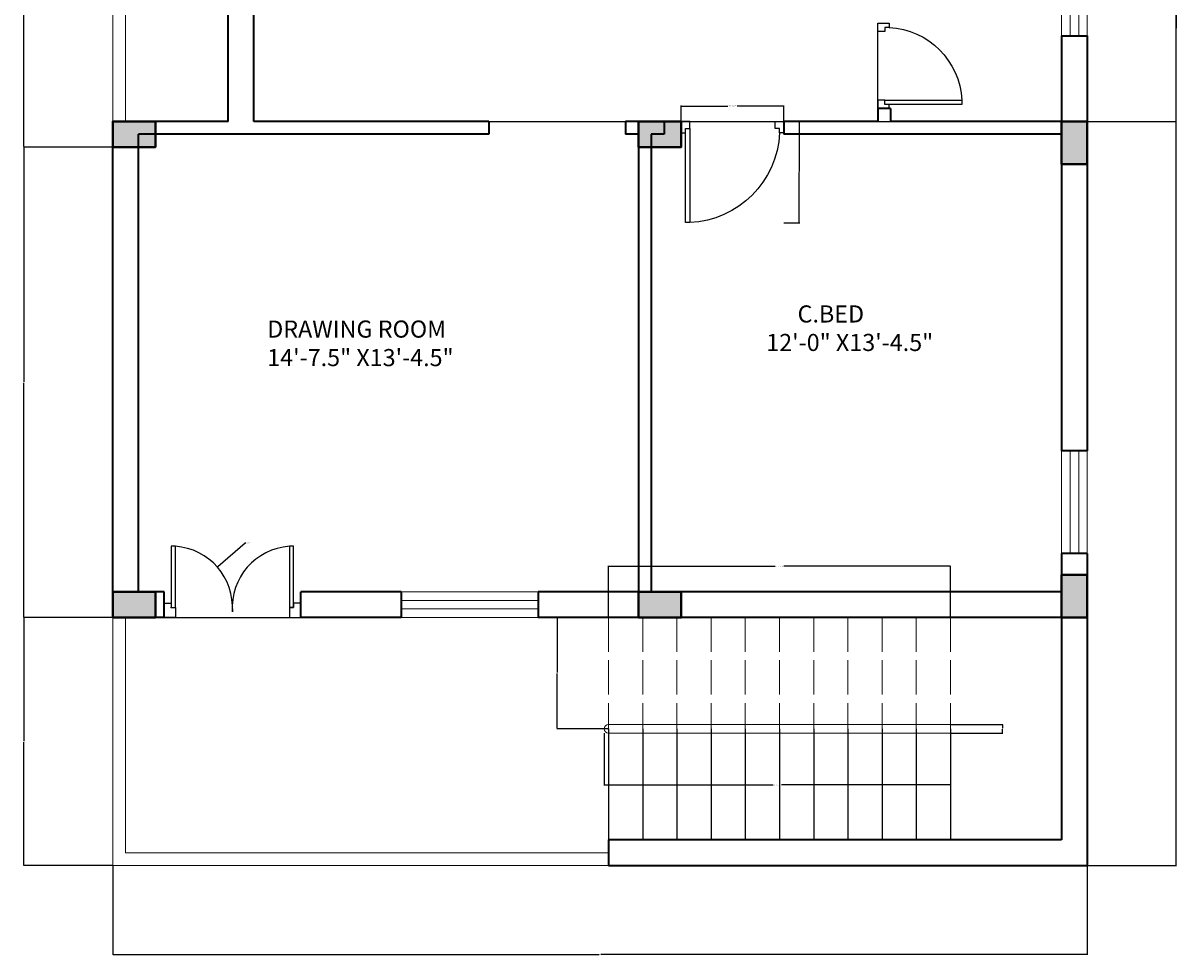
# Model space of a CAD drawing. Units: inches. Extents: x 810 to 2232, y 728 to 1827.
# Tile 5 of 6: x 1827 to 2232, y 1100 to 1426. Entities that reach past the tile are written whole.
import ezdxf

# ---------------------------------------------------------------- set-up
doc = ezdxf.new("R2010")
doc.units = ezdxf.units.IN
doc.linetypes.add('ACAD_ISO02W100', pattern=[15, 12, -3])
for name, color, linetype, lineweight in [('A-ANNO-DIMS', 2, 'Continuous', 18), ('A-AREA-IDEN', 50, 'Continuous', 18), ('A-FLOR-STRS-OVHD', 31, 'ACAD_ISO02W100', 18), ('column', 1, 'Continuous', 40), ('door', 150, 'Continuous', 25), ('railing', 233, 'Continuous', 18), ('staircase', 31, 'Continuous', 25), ('ventilator', 40, 'Continuous', 18), ('Wall', 7, 'Continuous', 35), ('window', 80, 'Continuous', 18)]:
    doc.layers.add(name, color=color, linetype=linetype, lineweight=lineweight)
doc.styles.get("Standard").update_dxf_attribs({"font": 'arial.ttf'})
doc.dimstyles.get("Standard").update_dxf_attribs({"dimtxt": 0.18, "dimasz": 0.18, "dimexe": 0.18, "dimexo": 0.0625, "dimgap": 0.09, "dimtad": 0, "dimtih": 1, "dimtoh": 1, "dimdec": 4, "dimzin": 0, "dimdsep": 46, "dimtxsty": 'Standard', "dimcen": 0.09, "dimadec": 0, "dimazin": 0, "dimtfac": 1, "dimtdec": 4, "dimtofl": 0, "dimtmove": 0, "dimatfit": 3, "dimfxl": 1, "dimtolj": 1, "dimtzin": 0, "dimarcsym": 0})

# ---------------------------------------------------------------- blocks, each defined once
blk = doc.blocks.new('MD')
at = {"layer": 'door'}
blk.add_line((1463.68, 2204.78), (1511.68, 2204.78), dxfattribs=at)
for points in [[(1466.18, 2208.28), (1467.68, 2208.28), (1467.68, 2229.78), (1466.18, 2229.78)], [(1507.68, 2208.28), (1509.18, 2208.28), (1509.18, 2229.78), (1507.68, 2229.78)]]:
    blk.add_lwpolyline(points, close=True, dxfattribs=at)
for points in [[(1467.68, 2204.78), (1463.68, 2204.78), (1463.68, 2209.78), (1466.18, 2209.78), (1466.18, 2208.28), (1467.68, 2208.28), (1467.68, 2204.78)], [(1507.68, 2204.78), (1511.68, 2204.78), (1511.68, 2209.78), (1509.18, 2209.78), (1509.18, 2208.28), (1507.68, 2208.28), (1507.68, 2204.78)]]:
    blk.add_lwpolyline(points, dxfattribs=at)
for centre, start, end in [((1466.18, 2208.28), 356.0091, 86.0091), ((1509.18, 2208.28), 93.9909, 183.9909)]:
    blk.add_arc(centre, 21.55, start, end, dxfattribs=at)
blk = doc.blocks.new('BD')
at = {"layer": 'door'}
blk.add_line((1349.9, 2199.58), (1385.9, 2199.58), dxfattribs=at)
blk.add_lwpolyline([(1351.4, 2202.08), (1352.9, 2202.08), (1352.9, 2235.08), (1351.4, 2235.08)], close=True, dxfattribs=at)
for points in [[(1352.9, 2199.58), (1349.9, 2199.58), (1349.9, 2203.58), (1351.4, 2203.58), (1351.4, 2202.08), (1352.9, 2202.08), (1352.9, 2199.58)], [(1382.9, 2199.58), (1385.9, 2199.58), (1385.9, 2203.58), (1384.4, 2203.58), (1384.4, 2202.08), (1382.9, 2202.08), (1382.9, 2199.58)]]:
    blk.add_lwpolyline(points, dxfattribs=at)
blk.add_arc((1351.4, 2202.08), 33.03, 2.6026, 87.3974, dxfattribs=at)
blk = doc.blocks.new('TD')
at = {"layer": 'door'}
blk.add_line((1594.06, 2210.18), (1624.06, 2210.18), dxfattribs=at)
blk.add_lwpolyline([(1595.56, 2212.68), (1597.06, 2212.68), (1597.06, 2239.68), (1595.56, 2239.68)], close=True, dxfattribs=at)
for points in [[(1597.06, 2210.18), (1594.06, 2210.18), (1594.06, 2214.18), (1595.56, 2214.18), (1595.56, 2212.68), (1597.06, 2212.68), (1597.06, 2210.18)], [(1621.06, 2210.18), (1624.06, 2210.18), (1624.06, 2214.18), (1622.56, 2214.18), (1622.56, 2212.68), (1621.06, 2212.68), (1621.06, 2210.18)]]:
    blk.add_lwpolyline(points, dxfattribs=at)
blk.add_arc((1595.56, 2212.68), 27.04, 3.1798, 86.8202, dxfattribs=at)
blk = doc.blocks.new('HW')
at = {"layer": 'window'}
for p, q in [((1851.89, 1931.95), (1887.89, 1931.95)), ((1851.89, 1928.95), (1887.89, 1928.95))]:
    blk.add_line(p, q, dxfattribs=at)
blk.add_lwpolyline([(1851.89, 1925.95), (1887.89, 1925.95), (1887.89, 1934.95), (1851.89, 1934.95)], close=True, dxfattribs=at)
blk = doc.blocks.new('BW')
at = {"layer": 'window'}
blk.add_blockref('HW', (0, 0), dxfattribs=at)
blk = doc.blocks.new('V')
at = {"layer": 'ventilator'}
for p, q in [((1926.2, 1912.67), (1950.2, 1912.67)), ((1926.2, 1909.67), (1950.2, 1909.67))]:
    blk.add_line(p, q, dxfattribs=at)
blk.add_lwpolyline([(1926.2, 1906.67), (1950.2, 1906.67), (1950.2, 1915.67), (1926.2, 1915.67)], close=True, dxfattribs=at)
blk = doc.blocks.new('DW')
at = {"layer": 'window'}
for p, q in [((1929.05, 1943.86), (1977.05, 1943.86)), ((1929.05, 1940.86), (1977.05, 1940.86))]:
    blk.add_line(p, q, dxfattribs=at)
blk.add_lwpolyline([(1929.05, 1937.86), (1977.05, 1937.86), (1977.05, 1946.86), (1929.05, 1946.86)], close=True, dxfattribs=at)
blk = doc.blocks.new('C1')
at = {"layer": 'column'}
h = blk.add_hatch(color=256, dxfattribs=at)
h.dxf.hatch_style = 1
h.paths.add_polyline_path([(431.83, 1717.82), (446.83, 1717.82), (446.83, 1726.82), (431.83, 1726.82)])
blk.add_lwpolyline([(431.83, 1717.82), (446.83, 1717.82), (446.83, 1726.82), (431.83, 1726.82)], close=True, dxfattribs=at)
blk = doc.blocks.new('STAIR-CENTRE-HANDRAIL')
for p, q in [((121.5, 3), (1.5, 3)), ((121.5, 0), (1.5, 0))]:
    blk.add_line(p, q)
blk.add_arc((1.5, 1.5), 1.5, 90, 270)
blk = doc.blocks.new('STAIR-FLIGHT-39IN')
for p, q in [((0, 39), (0, 0)), ((12, 39), (12, 0)), ((24, 39), (24, 0)), ((36, 39), (36, 0)), ((48, 39), (48, 0)), ((60, 39), (60, 0)), ((72, 39), (72, 0)), ((84, 39), (84, 0)), ((96, 39), (96, 0)), ((108, 39), (108, 0)), ((120, 39), (120, 0))]:
    blk.add_line(p, q)
blk = doc.blocks.new('STAIR-FLIGHT-39IN-OVERHEAD')
for p, q in [((0, 39), (0, 0)), ((12, 39), (12, 0)), ((24, 39), (24, 0)), ((36, 39), (36, 0)), ((48, 39), (48, 0)), ((60, 39), (60, 0)), ((72, 39), (72, 0)), ((84, 39), (84, 0)), ((96, 39), (96, 0)), ((108, 39), (108, 0)), ((120, 39), (120, 0))]:
    blk.add_line(p, q)
blk = doc.blocks.new('*D29')
at = {"layer": 'A-ANNO-DIMS', "color": 0, "lineweight": -2, "transparency": 16777216}
for p, q in [((2058.12, 1392.01), (2058.12, 1397.52)), ((2058.3, 1397.34), (2074.5, 1397.34)), ((2093.94, 1397.34), (2077.74, 1397.34)), ((2094.12, 1392.01), (2094.12, 1397.52))]:
    blk.add_line(p, q, dxfattribs=at)
at = {"layer": 'A-ANNO-DIMS', "color": 0, "transparency": 16777216}
for points in [[(2058.3, 1397.37), (2058.3, 1397.31), (2058.12, 1397.34)], [(2093.94, 1397.37), (2093.94, 1397.31), (2094.12, 1397.34)]]:
    blk.add_solid(points, dxfattribs=at)
at = {"layer": 'Defpoints', "color": 0, "transparency": 16777216}
for p in [(2094.12, 1397.34), (2058.12, 1391.94), (2094.12, 1391.94)]:
    blk.add_point(p, dxfattribs=at)
at = {"layer": 'A-ANNO-DIMS', "color": 0, "transparency": 16777216, "insert": (2076.12, 1397.34), "char_height": 0.18, "attachment_point": 5}
blk.add_mtext('\\A1;BEDROOM DOOR 36 TYP.', dxfattribs=at)
blk = doc.blocks.new('*D30')
at = {"layer": 'A-ANNO-DIMS', "color": 0, "lineweight": -2, "transparency": 16777216}
for p, q in [((2094.18, 1391.94), (2099.7, 1391.94)), ((2099.52, 1391.76), (2099.52, 1374.37)), ((2099.52, 1356.62), (2099.52, 1374.01)), ((2094.18, 1356.44), (2099.7, 1356.44))]:
    blk.add_line(p, q, dxfattribs=at)
at = {"layer": 'A-ANNO-DIMS', "color": 0, "transparency": 16777216}
for points in [[(2099.49, 1391.76), (2099.55, 1391.76), (2099.52, 1391.94)], [(2099.49, 1356.62), (2099.55, 1356.62), (2099.52, 1356.44)]]:
    blk.add_solid(points, dxfattribs=at)
at = {"layer": 'Defpoints', "color": 0, "transparency": 16777216}
for p in [(2094.12, 1391.94), (2094.12, 1356.44), (2099.52, 1356.44)]:
    blk.add_point(p, dxfattribs=at)
at = {"layer": 'A-ANNO-DIMS', "color": 0, "transparency": 16777216, "insert": (2099.52, 1374.19), "char_height": 0.18, "attachment_point": 5}
blk.add_mtext('\\A1;36 TYP.', dxfattribs=at)
blk = doc.blocks.new('*D51')
at = {"layer": 'A-ANNO-DIMS', "color": 0, "lineweight": -2, "transparency": 16777216}
for p, q in [((2031.12, 1177.38), (2031.12, 1159.04)), ((2152.62, 1177.38), (2152.62, 1159.04)), ((2031.3, 1159.22), (2090.4, 1159.22)), ((2152.44, 1159.22), (2093.33, 1159.22))]:
    blk.add_line(p, q, dxfattribs=at)
at = {"layer": 'A-ANNO-DIMS', "color": 0, "transparency": 16777216}
for points in [[(2031.3, 1159.25), (2031.3, 1159.19), (2031.12, 1159.22)], [(2152.44, 1159.25), (2152.44, 1159.19), (2152.62, 1159.22)]]:
    blk.add_solid(points, dxfattribs=at)
at = {"layer": 'Defpoints', "color": 0, "transparency": 16777216}
for p in [(2031.12, 1177.44), (2152.62, 1177.44), (2152.62, 1159.22)]:
    blk.add_point(p, dxfattribs=at)
at = {"layer": 'A-ANNO-DIMS', "color": 0, "transparency": 16777216, "insert": (2091.87, 1159.22), "char_height": 0.18, "attachment_point": 5}
blk.add_mtext('\\A1;CENTRE RAIL 122 TYP.', dxfattribs=at)
blk = doc.blocks.new('*D52')
at = {"layer": 'A-ANNO-DIMS', "color": 0, "lineweight": -2, "transparency": 16777216}
for p, q in [((2152.68, 1180.44), (2171.02, 1180.44)), ((2170.84, 1180.26), (2170.84, 1179.12)), ((2170.84, 1177.62), (2170.84, 1178.76)), ((2152.68, 1177.44), (2171.02, 1177.44))]:
    blk.add_line(p, q, dxfattribs=at)
at = {"layer": 'A-ANNO-DIMS', "color": 0, "transparency": 16777216}
for points in [[(2170.81, 1180.26), (2170.87, 1180.26), (2170.84, 1180.44)], [(2170.81, 1177.62), (2170.87, 1177.62), (2170.84, 1177.44)]]:
    blk.add_solid(points, dxfattribs=at)
at = {"layer": 'Defpoints', "color": 0, "transparency": 16777216}
for p in [(2152.62, 1180.44), (2170.84, 1180.44), (2152.62, 1177.44)]:
    blk.add_point(p, dxfattribs=at)
at = {"layer": 'A-ANNO-DIMS', "color": 0, "transparency": 16777216, "insert": (2170.84, 1178.94), "char_height": 0.18, "attachment_point": 5}
blk.add_mtext('\\A1;3 TYP.', dxfattribs=at)
blk = doc.blocks.new('*D57')
at = {"layer": 'A-ANNO-DIMS', "color": 0, "lineweight": -2, "transparency": 16777216}
for p, q in [((2032.62, 1218.01), (2032.62, 1236.12)), ((2032.8, 1235.94), (2091.07, 1235.94)), ((2152.44, 1235.94), (2094.16, 1235.94)), ((2152.62, 1218.01), (2152.62, 1236.12))]:
    blk.add_line(p, q, dxfattribs=at)
at = {"layer": 'A-ANNO-DIMS', "color": 0, "transparency": 16777216}
for points in [[(2032.8, 1235.97), (2032.8, 1235.91), (2032.62, 1235.94)], [(2152.44, 1235.97), (2152.44, 1235.91), (2152.62, 1235.94)]]:
    blk.add_solid(points, dxfattribs=at)
at = {"layer": 'Defpoints', "color": 0, "transparency": 16777216}
for p in [(2152.62, 1235.94), (2032.62, 1217.94), (2152.62, 1217.94)]:
    blk.add_point(p, dxfattribs=at)
at = {"layer": 'A-ANNO-DIMS', "color": 0, "transparency": 16777216, "insert": (2092.62, 1235.94), "char_height": 0.18, "attachment_point": 5}
blk.add_mtext('\\A1;FLIGHT ABOVE 120 TYP.', dxfattribs=at)
blk = doc.blocks.new('*D58')
at = {"layer": 'A-ANNO-DIMS', "color": 0, "lineweight": -2, "transparency": 16777216}
for p, q in [((2032.55, 1217.94), (2014.44, 1217.94)), ((2014.62, 1217.76), (2014.62, 1198.62)), ((2014.62, 1179.12), (2014.62, 1198.26)), ((2032.55, 1178.94), (2014.44, 1178.94))]:
    blk.add_line(p, q, dxfattribs=at)
at = {"layer": 'A-ANNO-DIMS', "color": 0, "transparency": 16777216}
for points in [[(2014.59, 1217.76), (2014.65, 1217.76), (2014.62, 1217.94)], [(2014.59, 1179.12), (2014.65, 1179.12), (2014.62, 1178.94)]]:
    blk.add_solid(points, dxfattribs=at)
at = {"layer": 'Defpoints', "color": 0, "transparency": 16777216}
for p in [(2014.62, 1217.94), (2032.62, 1217.94), (2032.62, 1178.94)]:
    blk.add_point(p, dxfattribs=at)
at = {"layer": 'A-ANNO-DIMS', "color": 0, "transparency": 16777216, "insert": (2014.62, 1198.44), "char_height": 0.18, "attachment_point": 5}
blk.add_mtext('\\A1;39 TYP.', dxfattribs=at)
blk = doc.blocks.new('*D66')
at = {"layer": 'A-ANNO-DIMS', "color": 0, "lineweight": -2, "transparency": 16777216}
for p, q in [((1858.62, 1130.88), (1858.62, 1099.61)), ((2200.62, 1130.88), (2200.62, 1099.61)), ((1858.8, 1099.79), (2029.33, 1099.79)), ((2200.44, 1099.79), (2029.9, 1099.79))]:
    blk.add_line(p, q, dxfattribs=at)
at = {"layer": 'A-ANNO-DIMS', "color": 0, "transparency": 16777216}
for points in [[(1858.8, 1099.82), (1858.8, 1099.76), (1858.62, 1099.79)], [(2200.44, 1099.82), (2200.44, 1099.76), (2200.62, 1099.79)]]:
    blk.add_solid(points, dxfattribs=at)
at = {"layer": 'Defpoints', "color": 0, "transparency": 16777216}
for p in [(1858.62, 1130.94), (2200.62, 1130.94), (2200.62, 1099.79)]:
    blk.add_point(p, dxfattribs=at)
at = {"layer": 'A-ANNO-DIMS', "color": 0, "transparency": 16777216, "insert": (2029.62, 1099.79), "char_height": 0.18, "attachment_point": 5}
blk.add_mtext('\\A1;342', dxfattribs=at)
blk = doc.blocks.new('*D67')
at = {"layer": 'A-ANNO-DIMS', "color": 0, "lineweight": -2, "transparency": 16777216}
for p, q in [((2200.68, 1751.94), (2231.95, 1751.94)), ((2231.77, 1751.76), (2231.77, 1441.62)), ((2231.77, 1131.12), (2231.77, 1441.26)), ((2200.68, 1130.94), (2231.95, 1130.94))]:
    blk.add_line(p, q, dxfattribs=at)
at = {"layer": 'A-ANNO-DIMS', "color": 0, "transparency": 16777216}
for points in [[(2231.74, 1751.76), (2231.8, 1751.76), (2231.77, 1751.94)], [(2231.74, 1131.12), (2231.8, 1131.12), (2231.77, 1130.94)]]:
    blk.add_solid(points, dxfattribs=at)
at = {"layer": 'Defpoints', "color": 0, "transparency": 16777216}
for p in [(2200.62, 1751.94), (2231.77, 1751.94), (2200.62, 1130.94)]:
    blk.add_point(p, dxfattribs=at)
at = {"layer": 'A-ANNO-DIMS', "color": 0, "transparency": 16777216, "insert": (2231.77, 1441.44), "char_height": 0.18, "attachment_point": 5}
blk.add_mtext('\\A1;621', dxfattribs=at)
blk = doc.blocks.new('*D68')
at = {"layer": 'A-ANNO-DIMS', "color": 0, "lineweight": -2, "transparency": 16777216}
for p, q in [((1858.55, 1217.94), (1827.29, 1217.94)), ((1827.47, 1217.76), (1827.47, 1174.62)), ((1827.47, 1131.12), (1827.47, 1174.26)), ((1858.55, 1130.94), (1827.29, 1130.94))]:
    blk.add_line(p, q, dxfattribs=at)
at = {"layer": 'A-ANNO-DIMS', "color": 0, "transparency": 16777216}
for points in [[(1827.44, 1217.76), (1827.5, 1217.76), (1827.47, 1217.94)], [(1827.44, 1131.12), (1827.5, 1131.12), (1827.47, 1130.94)]]:
    blk.add_solid(points, dxfattribs=at)
at = {"layer": 'Defpoints', "color": 0, "transparency": 16777216}
for p in [(1827.47, 1217.94), (1858.62, 1217.94), (1858.62, 1130.94)]:
    blk.add_point(p, dxfattribs=at)
at = {"layer": 'A-ANNO-DIMS', "color": 0, "transparency": 16777216, "insert": (1827.47, 1174.44), "char_height": 0.18, "attachment_point": 5}
blk.add_mtext('\\A1;87', dxfattribs=at)
blk = doc.blocks.new('*D69')
at = {"layer": 'A-ANNO-DIMS', "color": 0, "lineweight": -2, "transparency": 16777216}
for p, q in [((1858.55, 1382.94), (1827.29, 1382.94)), ((1827.47, 1382.76), (1827.47, 1300.62)), ((1827.47, 1218.12), (1827.47, 1300.26)), ((1858.55, 1217.94), (1827.29, 1217.94))]:
    blk.add_line(p, q, dxfattribs=at)
at = {"layer": 'A-ANNO-DIMS', "color": 0, "transparency": 16777216}
for points in [[(1827.44, 1382.76), (1827.5, 1382.76), (1827.47, 1382.94)], [(1827.44, 1218.12), (1827.5, 1218.12), (1827.47, 1217.94)]]:
    blk.add_solid(points, dxfattribs=at)
at = {"layer": 'Defpoints', "color": 0, "transparency": 16777216}
for p in [(1827.47, 1382.94), (1858.62, 1382.94), (1858.62, 1217.94)]:
    blk.add_point(p, dxfattribs=at)
at = {"layer": 'A-ANNO-DIMS', "color": 0, "transparency": 16777216, "insert": (1827.47, 1300.44), "char_height": 0.18, "attachment_point": 5}
blk.add_mtext('\\A1;165', dxfattribs=at)
blk = doc.blocks.new('*D70')
at = {"layer": 'A-ANNO-DIMS', "color": 0, "lineweight": -2, "transparency": 16777216}
for p, q in [((1858.55, 1558.44), (1827.29, 1558.44)), ((1827.47, 1558.26), (1827.47, 1470.87)), ((1827.47, 1383.12), (1827.47, 1470.51)), ((1858.55, 1382.94), (1827.29, 1382.94))]:
    blk.add_line(p, q, dxfattribs=at)
at = {"layer": 'A-ANNO-DIMS', "color": 0, "transparency": 16777216}
for points in [[(1827.44, 1558.26), (1827.5, 1558.26), (1827.47, 1558.44)], [(1827.44, 1383.12), (1827.5, 1383.12), (1827.47, 1382.94)]]:
    blk.add_solid(points, dxfattribs=at)
at = {"layer": 'Defpoints', "color": 0, "transparency": 16777216}
for p in [(1827.47, 1558.44), (1858.62, 1558.44), (1858.62, 1382.94)]:
    blk.add_point(p, dxfattribs=at)
at = {"layer": 'A-ANNO-DIMS', "color": 0, "transparency": 16777216, "insert": (1827.47, 1470.69), "char_height": 0.18, "attachment_point": 5}
blk.add_mtext('\\A1;175.5', dxfattribs=at)
blk = doc.blocks.new('*D74')
at = {"layer": 'A-ANNO-DIMS', "color": 0, "lineweight": -2, "transparency": 16777216}
for p, q in [((1908.18, 1457.19), (2231.95, 1457.19)), ((2231.77, 1457.01), (2231.77, 1424.75)), ((2231.77, 1392.12), (2231.77, 1424.39)), ((1908.18, 1391.94), (2231.95, 1391.94))]:
    blk.add_line(p, q, dxfattribs=at)
at = {"layer": 'A-ANNO-DIMS', "color": 0, "transparency": 16777216}
for points in [[(2231.74, 1457.01), (2231.8, 1457.01), (2231.77, 1457.19)], [(2231.74, 1392.12), (2231.8, 1392.12), (2231.77, 1391.94)]]:
    blk.add_solid(points, dxfattribs=at)
at = {"layer": 'Defpoints', "color": 0, "transparency": 16777216}
for p in [(1908.12, 1457.19), (2231.77, 1457.19), (1908.12, 1391.94)]:
    blk.add_point(p, dxfattribs=at)
at = {"layer": 'A-ANNO-DIMS', "color": 0, "transparency": 16777216, "insert": (2231.77, 1424.57), "char_height": 0.18, "attachment_point": 5}
blk.add_mtext('\\A1;65.25', dxfattribs=at)
blk = doc.blocks.new('*D95')
at = {"layer": 'A-ANNO-DIMS', "color": 0, "lineweight": -2, "transparency": 16777216}
for p, q in [((1905.14, 1244.07), (1895.52, 1235.7)), ((1905.32, 1244.07), (1905.14, 1244.07)), ((1879.03, 1221.44), (1879.21, 1221.44)), ((1879.12, 1221.35), (1879.12, 1221.53))]:
    blk.add_line(p, q, dxfattribs=at)
at = {"layer": 'A-ANNO-DIMS', "color": 0, "transparency": 16777216}
blk.add_solid([(1895.5, 1235.73), (1895.54, 1235.68), (1895.38, 1235.59)], dxfattribs=at)
at = {"layer": 'Defpoints', "color": 0, "transparency": 16777216}
for p in [(1895.38, 1235.59), (1879.12, 1221.44)]:
    blk.add_point(p, dxfattribs=at)
at = {"layer": 'A-ANNO-DIMS', "color": 0, "transparency": 16777216, "insert": (1906.06, 1244.07), "char_height": 0.18, "attachment_point": 5}
blk.add_mtext('\\A1;4X R21.552', dxfattribs=at)

msp = doc.modelspace()

# ---------------------------------------------------------------- linework, layer by layer
at = {"layer": 'railing'}
for p, q in [((1858.617, 1391.9426), (1858.617, 1558.4426)), ((1863.117, 1391.9426), (1863.117, 1558.4426)), ((1858.617, 1217.9426), (1858.617, 1130.9426)), ((1863.117, 1135.4426), (1863.117, 1217.9426)), ((2032.617, 1135.4426), (1863.117, 1135.4426)), ((2032.617, 1130.9426), (1858.617, 1130.9426))]:
    msp.add_line(p, q, dxfattribs=at)
at = {"layer": 'Wall'}
for p, q in [((1899.117, 1391.9426), (1899.117, 1457.1926)), ((1908.117, 1391.9426), (1908.117, 1457.1926)), ((2191.617, 1421.9426), (2200.617, 1421.9426)), ((2191.617, 1421.9426), (2191.617, 1391.9426)), ((2200.617, 1421.9426), (2200.617, 1276.4426)), ((2131.617, 1396.4426), (2127.117, 1396.4426)), ((2127.117, 1396.4426), (2127.117, 1391.9426)), ((2131.617, 1396.4426), (2131.617, 1391.9426)), ((1858.617, 1217.9426), (1858.617, 1391.9426)), ((1899.117, 1391.9426), (1858.617, 1391.9426)), ((1990.617, 1391.9426), (1908.117, 1391.9426)), ((1990.617, 1391.9426), (1990.617, 1387.4426)), ((2052.117, 1391.9426), (2038.617, 1391.9426)), ((2038.617, 1391.9426), (2038.617, 1387.4426)), ((2052.117, 1391.9426), (2052.117, 1387.4426)), ((2127.117, 1391.9426), (2094.117, 1391.9426)), ((2094.117, 1391.9426), (2094.117, 1387.4426)), ((2191.617, 1391.9426), (2131.617, 1391.9426)), ((1867.617, 1226.9426), (1867.617, 1387.4426)), ((1990.617, 1387.4426), (1867.617, 1387.4426)), ((2043.117, 1387.4426), (2038.617, 1387.4426)), ((2043.117, 1387.4426), (2043.117, 1226.9426)), ((2047.617, 1387.4426), (2047.617, 1226.9426)), ((2052.117, 1387.4426), (2047.617, 1387.4426)), ((2191.617, 1387.4426), (2094.117, 1387.4426)), ((2191.617, 1387.4426), (2191.617, 1276.4426)), ((2200.617, 1276.4426), (2191.617, 1276.4426)), ((2200.617, 1240.4426), (2191.617, 1240.4426)), ((2191.617, 1240.4426), (2191.617, 1226.9426)), ((2200.617, 1240.4426), (2200.617, 1130.9426)), ((1876.617, 1226.9426), (1867.617, 1226.9426)), ((1876.617, 1217.9426), (1876.617, 1226.9426)), ((1924.617, 1217.9426), (1924.617, 1226.9426)), ((1959.867, 1226.9426), (1924.617, 1226.9426)), ((1959.867, 1226.9426), (1959.867, 1217.9426)), ((2043.117, 1226.9426), (2007.867, 1226.9426)), ((2007.867, 1226.9426), (2007.867, 1217.9426)), ((2191.617, 1226.9426), (2047.617, 1226.9426)), ((1876.617, 1217.9426), (1858.617, 1217.9426)), ((1959.867, 1217.9426), (1924.617, 1217.9426)), ((2191.617, 1217.9426), (2007.867, 1217.9426)), ((2191.617, 1217.9426), (2191.617, 1139.9426)), ((2191.617, 1139.9426), (2032.617, 1139.9426)), ((2032.617, 1139.9426), (2032.617, 1130.9426)), ((2032.617, 1130.9426), (2200.617, 1130.9426))]:
    msp.add_line(p, q, dxfattribs=at)

# ---------------------------------------------------------------- block references
at = {"layer": 'A-FLOR-STRS-OVHD'}
msp.add_blockref('STAIR-FLIGHT-39IN-OVERHEAD', (2032.617, 1178.9426), dxfattribs=at)
at = {"layer": 'column'}
for p in [(1426.7867, -334.8728), (1611.2867, -334.8728), (1426.7867, -499.8728), (1611.2867, -499.8728)]:
    msp.add_blockref('C1', p, dxfattribs=at)
at = {"layer": 'column', "rotation": 90}
for p in [(3918.4324, 945.1124), (3918.4324, 786.1124)]:
    msp.add_blockref('C1', p, dxfattribs=at)
at = {"layer": 'door', "xscale": -1}
for name, p, rotation in [('TD', (-83.0636, -197.6185), 270), ('BD', (708.2171, 3591.5226), 180)]:
    msp.add_blockref(name, p, dxfattribs=dict(at, rotation=rotation))
at = {"layer": 'door'}
msp.add_blockref('MD', (412.9321, -986.8359), dxfattribs=at)
at = {"layer": 'railing'}
msp.add_blockref('STAIR-CENTRE-HANDRAIL', (2031.117, 1177.443), dxfattribs=at)
at = {"layer": 'staircase'}
msp.add_blockref('STAIR-FLIGHT-39IN', (2032.617, 1139.9426), dxfattribs=at)
at = {"layer": 'ventilator', "rotation": 270}
msp.add_blockref('V', (284.9489, 3372.1471), dxfattribs=at)
at = {"layer": 'window', "rotation": 270}
msp.add_blockref('BW', (265.6717, 3128.3341), dxfattribs=at)
at = {"layer": 'window'}
msp.add_blockref('DW', (30.8183, -719.9187), dxfattribs=at)

# ---------------------------------------------------------------- texts
at = {"layer": 'A-AREA-IDEN', "char_height": 6, "attachment_point": 1}
for s, width, insert in [('      C.BED\\P12\'-0" X13\'-4.5" ', 89.482208, (2087.9542, 1327.4241)), ('DRAWING ROOM\\P14\'-7.5" X13\'-4.5" ', 105.343087, (1912.8416, 1322.122))]:
    msp.add_mtext_dynamic_manual_height_columns(s, width=width, gutter_width=12.5, heights=[0], dxfattribs=dict(at, insert=insert))

# ---------------------------------------------------------------- dimensions: what is measured, and where the dimension line sits
at = {"layer": 'A-ANNO-DIMS'}
for base, p1, p2, override, picture, middle in [((2231.767, 1751.9426), (2200.617, 1130.9426), (2200.617, 1751.9426), {"dimdec": 0, "dimlfac": 1, "dimrnd": 0, "dimzin": 0, "dimdsep": 46, "dimlunit": 2}, '*D67', (2231.767, 1441.4426)), ((1827.467, 1558.4426), (1858.617, 1382.9426), (1858.617, 1558.4426), {"dimdec": 1, "dimlfac": 1, "dimrnd": 0, "dimzin": 0, "dimdsep": 46, "dimlunit": 2}, '*D70', (1827.467, 1470.6926)), ((2231.767, 1457.1926), (1908.117, 1391.9426), (1908.117, 1457.1926), {"dimdec": 2, "dimlfac": 1, "dimrnd": 0, "dimzin": 0, "dimdsep": 46, "dimlunit": 2}, '*D74', (2231.767, 1424.5676)), ((1827.467, 1382.9426), (1858.617, 1217.9426), (1858.617, 1382.9426), {"dimdec": 0, "dimlfac": 1, "dimrnd": 0, "dimzin": 0, "dimdsep": 46, "dimlunit": 2}, '*D69', (1827.467, 1300.4426)), ((1827.467, 1217.9426), (1858.617, 1130.9426), (1858.617, 1217.9426), {"dimdec": 0, "dimlfac": 1, "dimrnd": 0, "dimzin": 0, "dimdsep": 46, "dimlunit": 2}, '*D68', (1827.467, 1174.4426))]:
    dim = msp.add_linear_dim(base=base, p1=p1, p2=p2, angle=90, dimstyle='Standard', override=override, dxfattribs=at)
    dim.commit()
    dim.dimension.update_dxf_attribs({"geometry": picture, "text_midpoint": middle})
for base, p1, p2, text, picture, middle in [((2094.117, 1397.3426), (2058.117, 1391.9426), (2094.117, 1391.9426), 'BEDROOM DOOR <> TYP.', '*D29', (2076.117, 1397.3426)), ((2152.617, 1235.9426), (2032.617, 1217.9426), (2152.617, 1217.9426), 'FLIGHT ABOVE <> TYP.', '*D57', (2092.617, 1235.9426)), ((2152.6169726814, 1159.2176203011), (2031.1169726814, 1177.4426203011), (2152.6169726814, 1177.4426203011), 'CENTRE RAIL <> TYP.', '*D51', (2091.8669726814, 1159.2176203011))]:
    dim = msp.add_linear_dim(base=base, p1=p1, p2=p2, text=text, dimstyle='Standard', override={"dimdec": 0, "dimlfac": 1, "dimrnd": 0, "dimzin": 0, "dimdsep": 46, "dimlunit": 2}, dxfattribs=at)
    dim.commit()
    dim.dimension.update_dxf_attribs({"geometry": picture, "text_midpoint": middle})
for base, p1, p2, angle, picture, middle in [((2099.5169726814, 1356.4426203011), (2094.1169726814, 1391.9426203011), (2094.1169726814, 1356.4426203011), 270, '*D30', (2099.5169726814, 1374.1926203011)), ((2014.617, 1217.9426), (2032.617, 1178.9426), (2032.617, 1217.9426), 90, '*D58', (2014.617, 1198.4426)), ((2170.842, 1180.4426), (2152.617, 1177.4426), (2152.617, 1180.4426), 90, '*D52', (2170.842, 1178.9426))]:
    dim = msp.add_linear_dim(base=base, p1=p1, p2=p2, angle=angle, text='<> TYP.', dimstyle='Standard', override={"dimdec": 0, "dimlfac": 1, "dimrnd": 0, "dimzin": 0, "dimdsep": 46, "dimlunit": 2}, dxfattribs=at)
    dim.commit()
    dim.dimension.update_dxf_attribs({"geometry": picture, "text_midpoint": middle})
dim = msp.add_radius_dim(center=(1879.117, 1221.4426), mpoint=(1895.3801, 1235.5851), text='4X <>', dimstyle='Standard', override={"dimdec": 3, "dimlfac": 1, "dimrnd": 0, "dimzin": 0, "dimdsep": 46, "dimlunit": 2}, dxfattribs=at)
dim.commit()
dim.dimension.update_dxf_attribs({"geometry": '*D95', "text_midpoint": (1906.0639, 1244.0706), "dimtype": 164})
dim = msp.add_linear_dim(base=(2200.617, 1099.7926), p1=(1858.617, 1130.9426), p2=(2200.617, 1130.9426), dimstyle='Standard', override={"dimdec": 0, "dimlfac": 1, "dimrnd": 0, "dimzin": 0, "dimdsep": 46, "dimlunit": 2}, dxfattribs=at)
dim.commit()
dim.dimension.update_dxf_attribs({"geometry": '*D66', "text_midpoint": (2029.617, 1099.7926)})

doc.saveas('drawing.dxf')
